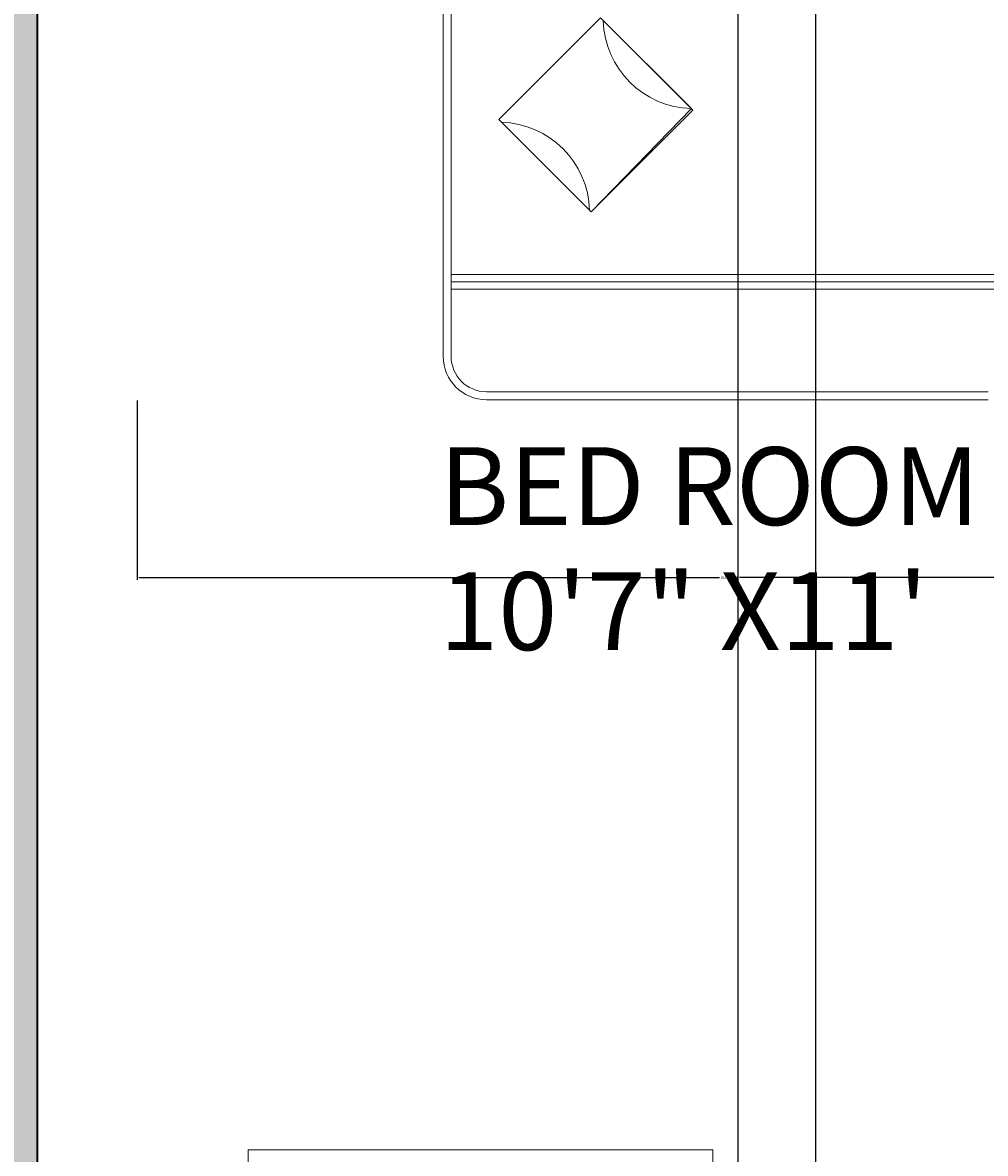
# Model space of a CAD drawing. Units: inches. Extents: x 2070 to 4408, y 1595 to 4269.
# Tile 11 of 20: x 2111 to 2185, y 2150 to 2238. Entities that reach past the tile are written whole.
import ezdxf

# ---------------------------------------------------------------- set-up
doc = ezdxf.new("R2010")
doc.units = ezdxf.units.IN
for name, color, linetype, lineweight in [('A-ANNO-DIMS', 2, 'Continuous', 18), ('A-AREA-IDEN', 7, 'Continuous', 18), ('A-DOOR', 4, 'Continuous', 18), ('A-FURN', 8, 'Continuous', 18), ('A-WALL', 7, 'Continuous', 35)]:
    doc.layers.add(name, color=color, linetype=linetype, lineweight=lineweight)
doc.layers.add('A-WALL-PATT', color=18, linetype='Continuous', lineweight=13, true_color=0x000000)
doc.styles.get("Standard").update_dxf_attribs({"font": 'arial.ttf'})
doc.dimstyles.get("Standard").update_dxf_attribs({"dimtxt": 0.18, "dimasz": 0.18, "dimexe": 0.18, "dimexo": 0.0625, "dimgap": 0.09, "dimtad": 0, "dimtih": 1, "dimtoh": 1, "dimdec": 4, "dimzin": 0, "dimdsep": 46, "dimtxsty": 'Standard', "dimcen": 0.09, "dimadec": 0, "dimazin": 0, "dimtfac": 1, "dimtdec": 4, "dimtofl": 0, "dimtmove": 0, "dimatfit": 3, "dimfxl": 1, "dimtolj": 1, "dimtzin": 0, "dimarcsym": 0})

# ---------------------------------------------------------------- blocks, each defined once
blk = doc.blocks.new('*U3')
for p, q in [((0, 0), (0, 6)), ((40, 0), (40, 6))]:
    blk.add_line(p, q)
blk.add_lwpolyline([(0, 0), (0, -40), (1.75, -40), (1.75, 0)], close=True)
blk.add_arc((0, 0), 40, 270, 0)
blk = doc.blocks.new('A$C18EB7ED0')
for p, q in [((0.7439, 1.8401), (0.7439, 0.1052)), ((0.7632, 1.8401), (0.7632, 0.1052)), ((0.8789, 0.6811), (1.1264, 0.9286)), ((0.8789, 0.6811), (1.1264, 0.9286)), ((1.1264, 0.9286), (1.3473, 0.7077)), ((1.1264, 0.9286), (1.3511, 0.7039)), ((1.3473, 0.7077), (1.1036, 0.4564)), ((1.3511, 0.7039), (1.1036, 0.4564)), ((1.1036, 0.4564), (0.8789, 0.6811)), ((1.1036, 0.4564), (0.8789, 0.6811)), ((0.7632, 0.3045), (2.155, 0.3045)), ((0.7632, 0.2865), (2.155, 0.2865)), ((0.7632, 0.2685), (2.155, 0.2685)), ((0.8491, 0.0193), (2.0691, 0.0193)), ((0.8491, 0), (2.0691, 0))]:
    blk.add_line(p, q)
for centre, radius, start, end in [((1.3534, 0.928), 0.2204, 181.5879, 268.4121), ((0.8795, 0.4541), 0.2204, 1.5879, 88.4121), ((0.8491, 0.1052), 0.1052, 180, 270), ((0.8491, 0.1052), 0.0859, 180, 270)]:
    blk.add_arc(centre, radius, start, end)
blk = doc.blocks.new('*D17')
at = {"layer": 'A-ANNO-DIMS', "color": 0, "lineweight": -2, "transparency": 16777216}
for p, q in [((2119.876, 2208.466), (2119.876, 2194.65)), ((2211.199, 2208.466), (2211.199, 2194.65)), ((2120.056, 2194.83), (2164.767, 2194.83)), ((2211.019, 2194.83), (2166.308, 2194.83))]:
    blk.add_line(p, q, dxfattribs=at)
at = {"layer": 'A-ANNO-DIMS', "color": 0, "transparency": 16777216}
for points in [[(2120.056, 2194.86), (2120.056, 2194.8), (2119.876, 2194.83)], [(2211.019, 2194.86), (2211.019, 2194.8), (2211.199, 2194.83)]]:
    blk.add_solid(points, dxfattribs=at)
at = {"layer": 'Defpoints', "color": 0, "transparency": 16777216}
for p in [(2119.876, 2208.528), (2211.199, 2208.528), (2211.199, 2194.83)]:
    blk.add_point(p, dxfattribs=at)
at = {"layer": 'A-ANNO-DIMS', "color": 0, "transparency": 16777216, "insert": (2165.538, 2194.83), "char_height": 0.18, "attachment_point": 5}
blk.add_mtext('\\A1;BED SET 91', dxfattribs=at)
blk = doc.blocks.new('*D24')
at = {"layer": 'A-ANNO-DIMS', "color": 0, "lineweight": -2, "transparency": 16777216}
for p, q in [((2103.133, 2291.4), (2069.836, 2291.4)), ((2070.016, 2291.22), (2070.016, 1960.081)), ((2070.016, 1628.58), (2070.016, 1959.718)), ((2336.133, 1628.4), (2069.836, 1628.4))]:
    blk.add_line(p, q, dxfattribs=at)
at = {"layer": 'A-ANNO-DIMS', "color": 0, "transparency": 16777216}
for points in [[(2069.986, 2291.22), (2070.046, 2291.22), (2070.016, 2291.4)], [(2069.986, 1628.58), (2070.046, 1628.58), (2070.016, 1628.4)]]:
    blk.add_solid(points, dxfattribs=at)
at = {"layer": 'Defpoints', "color": 0, "transparency": 16777216}
for p in [(2070.016, 2291.4), (2103.196, 2291.4), (2336.196, 1628.4)]:
    blk.add_point(p, dxfattribs=at)
at = {"layer": 'A-ANNO-DIMS', "color": 0, "transparency": 16777216, "insert": (2070.016, 1959.899), "char_height": 0.18, "attachment_point": 5}
blk.add_mtext('\\A1;663', dxfattribs=at)
blk = doc.blocks.new('*D28')
at = {"layer": 'A-ANNO-DIMS', "color": 0, "lineweight": -2, "transparency": 16777216}
for p, q in [((2166.196, 2000.462), (2166.196, 2324.76)), ((2172.196, 2000.462), (2172.196, 2324.76)), ((2166.376, 2324.579), (2169.047, 2324.579)), ((2172.016, 2324.579), (2169.345, 2324.579))]:
    blk.add_line(p, q, dxfattribs=at)
at = {"layer": 'A-ANNO-DIMS', "color": 0, "transparency": 16777216}
for points in [[(2166.376, 2324.61), (2166.376, 2324.55), (2166.196, 2324.579)], [(2172.016, 2324.61), (2172.016, 2324.55), (2172.196, 2324.579)]]:
    blk.add_solid(points, dxfattribs=at)
at = {"layer": 'Defpoints', "color": 0, "transparency": 16777216}
for p in [(2172.196, 2324.579), (2166.196, 2000.399), (2172.196, 2000.399)]:
    blk.add_point(p, dxfattribs=at)
at = {"layer": 'A-ANNO-DIMS', "color": 0, "transparency": 16777216, "insert": (2169.196, 2324.579), "char_height": 0.18, "attachment_point": 5}
blk.add_mtext('\\A1;6', dxfattribs=at)
blk = doc.blocks.new('*D31')
at = {"layer": 'A-ANNO-DIMS', "color": 0, "lineweight": -2, "transparency": 16777216}
for p, q in [((2112.196, 2000.462), (2112.196, 2324.76)), ((2166.196, 2000.462), (2166.196, 2324.76)), ((2112.376, 2324.579), (2138.977, 2324.579)), ((2166.016, 2324.579), (2139.415, 2324.579))]:
    blk.add_line(p, q, dxfattribs=at)
at = {"layer": 'A-ANNO-DIMS', "color": 0, "transparency": 16777216}
for points in [[(2112.376, 2324.61), (2112.376, 2324.55), (2112.196, 2324.579)], [(2166.016, 2324.61), (2166.016, 2324.55), (2166.196, 2324.579)]]:
    blk.add_solid(points, dxfattribs=at)
at = {"layer": 'Defpoints', "color": 0, "transparency": 16777216}
for p in [(2166.196, 2324.579), (2112.196, 2000.399), (2166.196, 2000.399)]:
    blk.add_point(p, dxfattribs=at)
at = {"layer": 'A-ANNO-DIMS', "color": 0, "transparency": 16777216, "insert": (2139.196, 2324.579), "char_height": 0.18, "attachment_point": 5}
blk.add_mtext('\\A1;54', dxfattribs=at)

msp = doc.modelspace()

# ---------------------------------------------------------------- hatches: boundary and pattern name
at = {"layer": 'A-WALL-PATT'}
h = msp.add_hatch(color=256, dxfattribs=at)
h.dxf.hatch_style = 1
h.paths.add_polyline_path([(2346.196, 2218.3995), (2346.196, 2282.3995), (2340.196, 2282.3995), (2340.196, 2212.3995), (2345.5866, 2212.3995), (2346.196, 2212.3995)], flags=0)
h.paths.add_polyline_path([(2245.196, 2282.3995), (2239.196, 2282.3995), (2239.196, 2186.3995), (2244.5866, 2186.3995), (2245.196, 2186.3995)], flags=0)
h.paths.add_polyline_path([(2340.196, 2230.6455), (2245.196, 2230.6455), (2245.196, 2224.6455), (2340.196, 2224.6455)], flags=0)
h.paths.add_polyline_path([(2245.196, 2150.3995), (2239.196, 2150.3995), (2164.4362, 2150.3995), (2164.4362, 2144.3995), (2239.196, 2144.3995), (2239.196, 2086.3995), (2239.196, 2067.2711), (2244.5866, 2067.2711), (2245.196, 2067.2711), (2245.196, 2144.3995)], flags=0)
h.paths.add_polyline_path([(2346.196, 2176.3995), (2340.196, 2176.3995), (2340.196, 2086.3995), (2346.196, 2086.3995), (2346.196, 2125.318)], flags=0)
h.paths.add_polyline_path([(2446.196, 2086.3995), (2346.196, 2086.3995), (2340.196, 2086.3995), (2340.196, 2080.3995), (2446.196, 2080.3995)], flags=0)
h.paths.add_polyline_path([(2455.196, 2291.3995), (2103.196, 2291.3995), (2103.196, 1699.3995), (2336.196, 1699.3995), (2336.196, 1628.3995), (2345.196, 1628.3995), (2446.196, 1628.3995), (2454.8846, 1628.3995), (2454.8846, 1699.3995)])
h.paths.add_polyline_path([(2446.196, 2282.3995), (2446.196, 2218.3995), (2446.196, 2212.3995), (2446.196, 2086.3995), (2446.196, 2080.3995), (2446.196, 1708.3995), (2446.196, 1637.3995), (2345.196, 1637.3995), (2345.196, 1699.3995), (2345.196, 1708.3995), (2336.196, 1708.3995), (2112.196, 1708.3995), (2112.196, 2282.3995), (2239.196, 2282.3995), (2245.196, 2282.3995), (2356.196, 2282.3995)], flags=16)
h.paths.add_polyline_path([(2245.196, 2150.3995), (2245.196, 2144.3995), (2245.196, 2067.2711), (2244.5866, 2067.2711), (2239.196, 2067.2711), (2239.196, 2065.6988), (2203.2929, 2065.6988, 0.4014527), (2239.196, 2031.3337), (2244.5866, 2031.3337), (2245.196, 2031.2711), (2245.196, 1924.1525), (2239.196, 1924.1525), (2239.196, 1922.5803), (2203.2929, 1922.5803, 0.4014527), (2239.196, 1888.2151), (2244.5866, 1888.2151), (2245.196, 1888.1525), (2245.196, 1748.3995), (2339.196, 1748.4621, -0.4014527), (2303.2929, 1782.8272), (2303.2585, 1782.8272), (2303.2585, 1784.3995), (2339.196, 1784.3995), (2339.196, 1877.2067), (2291.196, 1877.2067), (2291.196, 1883.2067), (2291.196, 1946.3995), (2291.196, 1952.3995), (2291.196, 2086.3995), (2297.196, 2086.3995), (2302.196, 2086.3995), (2302.196, 2081.0259), (2303.7633, 2081.0259), (2303.7633, 2080.3995), (2338.0148, 2080.3995, 0.0043713), (2338.0203, 2081.0259), (2338.0203, 2086.3995), (2340.196, 2086.3995), (2340.196, 2176.4621), (2345.5866, 2176.4621, 0.4014527), (2381.4896, 2210.8272), (2345.5866, 2210.8272), (2345.5866, 2212.3995), (2340.196, 2212.3995), (2340.196, 2224.6455), (2245.196, 2224.6455), (2245.196, 2186.3995), (2244.5866, 2186.3995), (2239.196, 2186.3995), (2239.196, 2184.8272), (2203.2929, 2184.8272, 0.4014527), (2239.196, 2150.4621), (2244.5866, 2150.4621)], flags=0)
h.paths.add_polyline_path([(2346.196, 2282.3995), (2346.196, 2218.3995), (2377.1813, 2218.3995), (2377.1813, 2212.3995), (2346.196, 2212.3995), (2345.5866, 2212.3995), (2340.196, 2212.3995), (2340.196, 2224.6455), (2245.196, 2224.6455), (2245.196, 2230.6455), (2245.196, 2282.3995), (2292.696, 2256.5225), (2340.196, 2282.3995)], flags=0)
h.paths.add_polyline_path([(2346.196, 2086.3995), (2340.196, 2086.3995), (2340.196, 2080.3995), (2446.196, 2080.3995), (2431.196, 2016.3995), (2446.196, 1952.3995), (2412.196, 1952.3995), (2412.196, 2080.3995), (2340.196, 2080.3995), (2340.196, 2086.3995), (2340.196, 2176.3995), (2346.196, 2176.3995), (2346.196, 2125.318)], flags=0)
h.paths.add_polyline_path([(2186.508, 2270.0471, -0.0375529), (2186.9712, 2269.8581), (2186.9164, 2270.112, -0.0275912)], flags=0)
h.paths.add_polyline_path([(2183.955, 2273.7766, 1), (2188.2945, 2273.7766, 1)], flags=0)
h.paths.add_polyline_path([(2142.5261, 2274.6158, -0.0370754), (2142.5672, 2275.1696), (2142.5672, 2276.826), (2119.8759, 2276.826), (2119.8759, 2263.0962), (2140.4332, 2263.0962), (2142.5672, 2263.0962), (2142.5672, 2274.0621, -0.0370754)], flags=0)
h.paths.add_polyline_path([(2209.8974, 2263.0962), (2209.8974, 2262.2079), (2190.8042, 2262.2079), (2190.8042, 2263.0962)], flags=0)
h.paths.add_polyline_path([(2210.6382, 2276.1833), (2210.6382, 2263.9844), (2190.2185, 2263.9844), (2190.2185, 2276.1833)], flags=0)
h.paths.add_polyline_path([(2188.4362, 2273.7766, -1), (2183.8133, 2273.7766, -1)], flags=0)
h.paths.add_polyline_path([(2245.196, 2150.3995), (2245.196, 2144.3995), (2245.196, 2067.2711), (2239.196, 2067.2711), (2239.196, 2080.3995), (2172.196, 2080.3995), (2172.196, 2000.3995), (2239.196, 2000.3995), (2239.196, 1940.3995), (2159.0187, 1940.3995), (2123.0187, 1940.3995), (2112.196, 1940.3995), (2112.196, 1946.3995), (2123.0187, 1946.3995), (2123.0187, 1982.2238), (2124.586, 1982.2238), (2124.586, 1982.1895, -0.4014527), (2158.8429, 1946.3995), (2159.0187, 1946.3995), (2239.196, 1946.3995), (2239.196, 1994.3995), (2112.196, 1994.3995), (2112.196, 2000.3995), (2139.196, 2040.3995), (2112.196, 2080.3995), (2112.196, 2086.3995), (2239.196, 2086.3995), (2239.196, 2144.3995), (2209.5809, 2144.3995), (2209.5809, 2136.3995), (2203.0809, 2136.3995), (2205.0809, 2130.3996, -0.7025712), (2199.081, 2116.3995, -0.7025621), (2193.0809, 2130.3994), (2195.0809, 2136.3995), (2192.0809, 2136.3995), (2192.0809, 2134.8995), (2189.0809, 2134.8995), (2189.0809, 2135.8995), (2191.0809, 2135.8995), (2191.0809, 2136.3995), (2188.5809, 2136.3995), (2188.5809, 2144.3995), (2164.2481, 2144.3995, -0.3938585), (2130.0035, 2109.5491), (2130.0035, 2109.5147), (2128.4362, 2109.5147), (2128.4362, 2144.3995), (2112.196, 2144.3995), (2112.196, 2150.3995), (2128.4362, 2150.3995), (2128.4362, 2150.7127), (2164.4362, 2150.7127), (2164.4362, 2150.3995), (2239.196, 2150.3995)], flags=0)
h.paths.add_polyline_path([(2188.2075, 2266.8735), (2188.2075, 2211.8632, -0.4142136), (2185.4833, 2209.1391), (2146.7995, 2209.1391, -0.4142136), (2144.0754, 2211.8632), (2144.0754, 2266.8735, -0.4142136), (2146.7995, 2269.5976), (2185.4833, 2269.5976, -0.4142136)], flags=0)
h.paths.add_polyline_path([(2185.0844, 2273.7766, -1), (2187.1651, 2273.7766, -1)], flags=0)
h.paths.add_polyline_path([(2182.0486, 2259.2932), (2168.0953, 2259.2932), (2168.0953, 2260.8424), (2163.7261, 2260.8424), (2163.7261, 2259.2932), (2149.7727, 2259.2932), (2149.7727, 2266.3352), (2163.7261, 2266.3352), (2163.7261, 2261.9839), (2168.0953, 2261.9839), (2168.0953, 2266.3352), (2182.0486, 2266.3352)], flags=0)
h.paths.add_polyline_path([(2148.2585, 2250.2051), (2153.0615, 2241.8861, 0.3980705)], flags=0)
h.paths.add_polyline_path([(2162.7572, 2247.2885), (2153.1461, 2241.7396), (2148.1083, 2250.4653), (2157.7194, 2256.0142)], flags=0)
h.paths.add_polyline_path([(2162.6726, 2247.4351, -0.392862), (2157.8415, 2255.6313), (2157.6431, 2255.6313), (2157.8696, 2255.7541)], flags=0)
h.paths.add_polyline_path([(2164.2604, 2145.339), (2164.4362, 2144.3995), (2164.4362, 2150.3995), (2164.2604, 2150.7127)], flags=0)
h.paths.add_polyline_path([(2208.5809, 2142.6495), (2208.5809, 2138.3995, -0.4142136), (2207.8309, 2137.3995), (2190.5809, 2137.3995, -0.4142136), (2189.5809, 2138.1495), (2189.5809, 2142.3995, -0.4142136), (2190.3309, 2143.3995), (2207.5809, 2143.3995, -0.4142136)], flags=0)
h.paths.add_polyline_path([(2147.957, 2229.9119), (2154.7494, 2223.1195, 0.3980705)], flags=0)
h.paths.add_polyline_path([(2162.7165, 2230.8473), (2154.8691, 2222.9998), (2147.7446, 2230.1244), (2155.592, 2237.9718)], flags=0)
h.paths.add_polyline_path([(2162.5969, 2230.9669, -0.3980705), (2155.8044, 2237.7594)], flags=0)
h.paths.add_polyline_path([(2391.8776, 2049.9192), (2408.5766, 2049.9192), (2408.5766, 2033.2202), (2408.5766, 1983.123), (2408.5766, 1966.4239), (2391.8776, 1966.4239), (2391.8776, 1983.123), (2341.7804, 1983.123), (2341.7804, 2033.2202), (2391.8776, 2033.2202)], flags=0)
h.paths.add_polyline_path([(2144.1055, 2274.6158, 1), (2148.445, 2274.6158, 1)], flags=0)
h.paths.add_polyline_path([(2148.5867, 2274.6158, -1), (2143.9638, 2274.6158, -1)], flags=0)
h.paths.add_polyline_path([(2145.2349, 2274.6158, -1), (2147.3156, 2274.6158, -1)], flags=0)
edge = h.paths.add_edge_path(flags=0)
edge.add_ellipse((2400.5951, 2040.9436), major_axis=(-4.5109, 0), ratio=0.9754478, start_angle=180, end_angle=270, ccw=False)
edge.add_ellipse((2400.5951, 2040.9436), major_axis=(-4.5109, 0), ratio=0.9754478, start_angle=90, end_angle=180, ccw=False)
edge.add_ellipse((2400.5951, 2040.9436), major_axis=(-4.5109, 0), ratio=0.9754478, start_angle=0, end_angle=90, ccw=False)
edge.add_ellipse((2400.5951, 2040.9436), major_axis=(-4.5109, 0), ratio=0.9754478, start_angle=270, end_angle=360, ccw=False)
h.paths.add_polyline_path([(2199.0809, 2117.3995, -0.7345297), (2195.0809, 2130.3995), (2203.081, 2130.3995, -0.7345333)], flags=0)
h.paths.add_polyline_path([(2141.9147, 2276.0353), (2141.9147, 2263.9844), (2120.4685, 2263.9844), (2120.4685, 2276.0353)], flags=0)
h.paths.add_polyline_path([(2138.4481, 2273.4072), (2138.4481, 2266.7226), (2133.2801, 2266.7226), (2133.2801, 2273.4072)], flags=0)
h.paths.add_polyline_path([(2137.9691, 2272.9175), (2137.9691, 2272.204), (2135.4229, 2272.204), (2135.4229, 2271.6329), (2135.3221, 2270.1051), (2135.3221, 2269.0265), (2135.4229, 2268.6811), (2135.4229, 2267.2011), (2133.7212, 2267.2011), (2133.7212, 2268.6811), (2133.7983, 2269.9587), (2133.7983, 2271.2758), (2133.7212, 2271.6329), (2133.7212, 2273.0065), (2135.717, 2273.0065), (2135.717, 2272.9175)], flags=0)
h.paths.add_polyline_path([(2137.9215, 2271.8264), (2137.9215, 2271.3786), (2137.5182, 2271.3786), (2136.9355, 2271.3786), (2136.3529, 2271.3786), (2135.7703, 2271.3786), (2135.7703, 2271.8264), (2136.1736, 2271.8264), (2136.7562, 2271.8264), (2137.3389, 2271.8264)], flags=0)
h.paths.add_polyline_path([(2137.9215, 2271.692), (2137.5182, 2271.692), (2136.9355, 2271.513), (2137.3389, 2271.513)], flags=0)
h.paths.add_polyline_path([(2136.3529, 2271.692), (2135.7703, 2271.513), (2136.1736, 2271.513), (2136.7562, 2271.692)], flags=0)
h.paths.add_polyline_path([(2137.9215, 2271.513), (2137.5182, 2271.513), (2136.7562, 2271.747), (2136.7562, 2271.692), (2137.3389, 2271.692)], flags=0)
h.paths.add_polyline_path([(2137.8207, 2270.4664), (2137.8207, 2270.0971), (2137.8207, 2269.627), (2137.8207, 2269.1569), (2137.8207, 2268.6868), (2137.3837, 2268.6868), (2136.6442, 2268.6868), (2135.9271, 2268.6868), (2135.9271, 2269.0562), (2135.9271, 2269.5263), (2135.9271, 2269.9963), (2135.9271, 2270.4664), (2136.3641, 2270.4664), (2137.0812, 2270.4664)], flags=0)
h.paths.add_polyline_path([(2137.3837, 2269.627), (2137.8207, 2269.627), (2137.8207, 2269.5263), (2137.3837, 2269.5263), (2137.3837, 2269.1569), (2137.8207, 2269.1569), (2137.3837, 2269.0562), (2137.3837, 2268.6868), (2137.0812, 2268.6868), (2137.0812, 2269.0562), (2136.6442, 2269.0562), (2136.6442, 2268.6868), (2136.3641, 2268.6868), (2136.3641, 2269.0562), (2135.9271, 2269.0562), (2135.9271, 2269.1569), (2136.3641, 2269.1569), (2136.3641, 2269.5263), (2135.9271, 2269.5263), (2135.9271, 2269.627), (2136.3641, 2269.627), (2136.3641, 2269.9963), (2135.9271, 2269.9963), (2136.3641, 2270.0971), (2136.3641, 2270.4664), (2136.6442, 2270.4664), (2136.6442, 2270.0971), (2137.0812, 2270.0971), (2137.0812, 2270.4664), (2137.3837, 2270.4664), (2137.3837, 2270.0971), (2137.8207, 2270.0971), (2137.3837, 2269.9963)], flags=0)
h.paths.add_polyline_path([(2137.5182, 2271.8264), (2137.5182, 2271.692), (2137.3389, 2271.3786), (2137.3389, 2271.513)], flags=0)
h.paths.add_polyline_path([(2137.8179, 2267.8138), (2137.8179, 2267.6879), (2137.1876, 2267.6879), (2136.4733, 2267.6879), (2135.759, 2267.6879), (2135.759, 2267.8138), (2136.3893, 2267.8138), (2137.1036, 2267.8138)], flags=0)
h.paths.add_polyline_path([(2137.0812, 2269.9963), (2137.0812, 2269.627), (2137.0812, 2269.1569), (2136.6442, 2269.1569), (2136.6442, 2269.5263), (2136.6442, 2269.9963)], flags=0)
h.paths.add_polyline_path([(2136.3529, 2271.8264), (2136.3529, 2271.692), (2136.1736, 2271.3786), (2136.1736, 2271.513)], flags=0)
h.paths.add_polyline_path([(2136.4733, 2267.8138), (2136.4733, 2267.6879), (2136.3893, 2267.6879), (2136.3893, 2267.8138)], flags=0)
h.paths.add_polyline_path([(2407.9087, 2032.5522), (2407.9087, 1983.7909), (2359.81, 1983.7909, -0.0091279), (2359.0575, 1983.7909), (2342.4483, 1983.7909), (2342.4483, 2032.5522)], flags=0)
h.paths.add_polyline_path([(2389.1838, 2023.1358), (2353.7856, 2023.1358), (2353.7856, 1985.4867, -0.0921038), (2350.2788, 1988.655), (2350.2788, 2026.6426), (2389.1838, 2026.6426)], flags=0)
h.paths.add_polyline_path([(2352.6166, 2024.3048), (2351.4477, 2024.3048), (2351.4477, 2025.4737), (2352.6166, 2025.4737)], flags=0)
h.paths.add_polyline_path([(2399.6319, 2026.7589), (2404.3661, 2026.7589, -0.4142136), (2407.0379, 2024.087), (2407.0379, 2013.4908, -0.4142136), (2404.3661, 2010.819), (2399.6319, 2010.819, -0.4142136), (2396.96, 2013.4908), (2396.96, 2024.087, -0.4142136)], flags=0)
h.paths.add_polyline_path([(2399.6319, 2026.0909), (2404.3661, 2026.0909, -0.4142136), (2406.37, 2024.087), (2406.37, 2013.4908, -0.4142136), (2404.3661, 2011.487), (2399.6319, 2011.487, -0.4142136), (2397.628, 2013.4908), (2397.628, 2024.087, -0.4142136)], flags=0)
h.paths.add_polyline_path([(2399.6319, 2002.3217), (2404.3661, 2002.3217, -0.4142136), (2407.0379, 1999.6498), (2407.0379, 1989.0536, -0.4142136), (2404.3661, 1986.3818), (2399.6319, 1986.3818, -0.4142136), (2396.96, 1989.0536), (2396.96, 1999.6498, -0.4142136)], flags=0)
h.paths.add_polyline_path([(2399.6319, 2001.6537), (2404.3661, 2001.6537, -0.4142136), (2406.37, 1999.6498), (2406.37, 1989.0536, -0.4142136), (2404.3661, 1987.0497), (2399.6319, 1987.0497, -0.4142136), (2397.628, 1989.0536), (2397.628, 1999.6498, -0.4142136)], flags=0)
edge = h.paths.add_edge_path(flags=0)
edge.add_ellipse((2400.5951, 1975.3996), major_axis=(-4.5109, 0), ratio=0.9754478, start_angle=-180, end_angle=-90, ccw=False)
edge.add_ellipse((2400.5951, 1975.3996), major_axis=(-4.5109, 0), ratio=0.9754478, start_angle=90, end_angle=180, ccw=False)
edge.add_ellipse((2400.5951, 1975.3996), major_axis=(-4.5109, 0), ratio=0.9754478, start_angle=0, end_angle=90, ccw=False)
edge.add_ellipse((2400.5951, 1975.3996), major_axis=(-4.5109, 0), ratio=0.9754478, start_angle=-90, end_angle=0, ccw=False)
h.paths.add_polyline_path([(2345.196, 1910.3995), (2366.4386, 1910.3995), (2366.4386, 1925.4555), (2392.3856, 1925.4555), (2392.3856, 1933.5025), (2400.1399, 1925.4555), (2392.3856, 1919.8795), (2392.3856, 1925.4555), (2366.4386, 1925.4555), (2366.4386, 1910.3995), (2381.196, 1910.3995), (2405.196, 1910.3995), (2405.196, 1898.3995), (2446.196, 1898.3995), (2446.196, 1886.3995), (2405.196, 1886.3995), (2405.196, 1874.3995), (2446.196, 1874.3995), (2446.196, 1862.3995), (2405.196, 1862.3995), (2405.196, 1850.3995), (2446.196, 1850.3995), (2446.196, 1838.3995), (2405.196, 1838.3995), (2405.196, 1826.3995), (2446.196, 1826.3995), (2446.196, 1814.3995), (2405.196, 1814.3995), (2405.196, 1802.3995), (2446.196, 1802.3995), (2446.196, 1798.3995), (2446.196, 1792.3995), (2405.196, 1792.3995), (2405.196, 1910.3995), (2381.196, 1910.3995), (2381.196, 1792.3995), (2345.196, 1792.3995)], flags=0)
h.paths.add_polyline_path([(2333.0944, 1863.3993, -0.4142136), (2334.7225, 1861.7712), (2334.7225, 1859.329), (2335.2653, 1859.329, -0.4142136), (2337.4361, 1857.1582), (2337.4361, 1843.862, -0.4142136), (2335.2653, 1841.6911, -0.4142136), (2337.4361, 1839.5203), (2337.4361, 1827.5808, -0.4142136), (2335.2653, 1825.41, -0.4142136), (2337.4361, 1823.2392), (2337.4361, 1808.5862, -0.4142136), (2335.2653, 1806.4153), (2334.7225, 1806.4153), (2334.7225, 1803.9732, -0.4142136), (2333.0944, 1802.3451), (2317.356, 1802.3451), (2317.0846, 1802.3451, -0.4142136), (2315.7279, 1803.7018), (2315.7279, 1803.8646), (2313.8284, 1803.8646, -0.4142136), (2311.6576, 1806.0354), (2311.6576, 1823.2015, -0.395976), (2313.6834, 1825.3765, -0.433848), (2311.6576, 1827.2718), (2311.6576, 1839.761, -0.4142136), (2313.5571, 1841.6604), (2313.8284, 1841.6604), (2333.8159, 1841.6604, -0.0421362), (2334.1798, 1841.6911, -0.4142136), (2332.009, 1843.862), (2332.009, 1857.1582, -0.4142136), (2334.1798, 1859.329), (2317.356, 1859.329), (2317.0846, 1859.329, -0.4142136), (2315.7279, 1860.6858), (2315.7279, 1862.0426, -0.4142136), (2317.0846, 1863.3993), (2317.356, 1863.3993)], flags=0)
h.paths.add_polyline_path([(2208.8475, 1848.9818), (2208.8475, 1840.9741, -0.4142136), (2207.0458, 1839.1724), (2206.5453, 1839.1721), (2206.5453, 1838.7218, -0.4098586), (2204.7704, 1836.9203), (2183.7501, 1836.9203, -0.418582), (2181.9216, 1838.7218), (2181.9216, 1839.1721), (2181.421, 1839.1724, -0.4142136), (2179.6193, 1840.9741), (2179.6193, 1848.6817, -0.4406442), (2185.1126, 1854.9874), (2203.3852, 1854.9874, -0.4570796)], flags=0)
h.paths.add_polyline_path([(2204.243, 1848.4815), (2204.243, 1848.4815, 0.4172533), (2202.2204, 1850.4833), (2186.2049, 1850.4833, 0.4111805), (2184.2237, 1848.4815), (2184.2237, 1848.4815, -0.4111807), (2186.2049, 1850.4833), (2202.2204, 1850.4833, -0.4172531)], flags=0)
h.paths.add_polyline_path([(2234.7177, 1830.228), (2234.7176, 1781.6047, -0.4142136), (2233.4381, 1780.3252), (2218.6064, 1780.3252, -0.4142136), (2217.8387, 1781.0929), (2217.8387, 1783.3961, -0.4142136), (2218.6064, 1784.1639), (2218.6065, 1796.9595, -0.4142136), (2219.886, 1798.239, -0.4142136), (2218.6065, 1799.5186), (2218.6065, 1812.3142, -0.4142136), (2219.8861, 1813.5938, -0.4142136), (2218.6065, 1814.8733), (2218.6065, 1827.6689, -0.4142136), (2217.8388, 1828.4367), (2217.8388, 1830.7399, -0.4142136), (2218.6065, 1831.5076), (2233.4382, 1831.5076, -0.4142136)], flags=0)
h.paths.add_polyline_path([(2230.6344, 1827.6689, -0.4142136), (2231.4021, 1826.9012), (2231.4021, 1784.9316, -0.4142136), (2230.6343, 1784.1639), (2221.1853, 1784.1639), (2221.1853, 1827.6689)], flags=0)
h.paths.add_polyline_path([(2222.7208, 1798.239), (2221.6971, 1798.239), (2221.6971, 1813.5938), (2222.7208, 1813.5938)], flags=0)
h.paths.add_polyline_path([(2206.5453, 1773.935), (2206.5453, 1773.4848), (2206.9457, 1773.4848), (2207.0458, 1773.4845, -0.4142136), (2208.8475, 1771.6827), (2208.8475, 1763.675, -0.4422243), (2203.6505, 1757.6695), (2185.3851, 1757.6695, -0.455084), (2179.6193, 1763.9752), (2179.6193, 1771.6827, -0.4142136), (2181.421, 1773.4845), (2181.421, 1773.4848), (2181.9216, 1773.4848), (2181.9216, 1773.935, -0.4098586), (2183.6965, 1775.7366), (2204.7167, 1775.7366, -0.418582)], flags=0)
h.paths.add_polyline_path([(2202.2619, 1762.1736), (2186.2464, 1762.1736, -0.4172531), (2184.2237, 1764.1754), (2184.2237, 1764.1754, 0.4172533), (2186.2464, 1762.1736), (2202.2619, 1762.1736, 0.4111805), (2204.243, 1764.1754), (2204.243, 1764.1754, -0.4111807)], flags=0)
h.paths.add_polyline_path([(2313.0034, 1713.1906), (2312.997, 1713.1697), (2313.0123, 1713.1612)], flags=0)
h.paths.add_polyline_path([(2305.7314, 1721.0488), (2305.6257, 1721.1994), (2305.4853, 1721.084)], flags=0)
h.paths.add_polyline_path([(2307.5562, 1726.1427), (2307.6186, 1726.1026), (2307.5737, 1726.0477), (2308.5692, 1720.6434), (2310.5345, 1721.2985), (2310.5721, 1721.411), (2310.6958, 1721.3523), (2313.8453, 1722.4021), (2314.9351, 1723.8033), (2314.9294, 1723.9165), (2315.0028, 1723.8903), (2313.874, 1722.4389), (2313.8697, 1722.4102), (2308.5692, 1720.6434), (2308.9864, 1720.122), (2309.0665, 1720.0971), (2309.053, 1720.0387), (2310.9235, 1717.7005), (2311.4182, 1717.6259), (2311.2918, 1717.2402), (2312.0655, 1716.2731), (2312.1081, 1716.2606), (2312.0969, 1716.2339), (2308.5692, 1720.6434), (2305.2249, 1717.745), (2305.232, 1717.704), (2305.1665, 1717.6944), (2308.5692, 1720.6434)], flags=0)
h.paths.add_polyline_path([(2288.2072, 1714.3431), (2288.2008, 1714.3222), (2288.216, 1714.3137)], flags=0)
h.paths.add_polyline_path([(2280.9352, 1722.2013), (2280.8295, 1722.3519), (2280.689, 1722.2365)], flags=0)
h.paths.add_polyline_path([(2282.76, 1727.2952), (2282.8224, 1727.2551), (2282.7775, 1727.2002), (2283.773, 1721.7959), (2285.7383, 1722.451), (2285.7759, 1722.5635), (2285.8995, 1722.5048), (2289.0491, 1723.5546), (2290.1389, 1724.9558), (2290.1332, 1725.069), (2290.2065, 1725.0428), (2289.0777, 1723.5915), (2289.0735, 1723.5628), (2283.773, 1721.7959), (2284.1901, 1721.2745), (2284.2703, 1721.2496), (2284.2567, 1721.1913), (2286.1273, 1718.8531), (2286.622, 1718.7785), (2286.4956, 1718.3927), (2287.2692, 1717.4256), (2287.3119, 1717.4131), (2287.3006, 1717.3864), (2283.773, 1721.7959), (2280.4286, 1718.8975), (2280.4357, 1718.8565), (2280.3703, 1718.8469), (2283.773, 1721.7959)], flags=0)
h.paths.add_polyline_path([(2302.0672, 1721.8694), (2301.8205, 1721.8572), (2301.7578, 1722.1787), (2299.415, 1724.5215), (2299.103, 1724.4694), (2299.0662, 1724.8703)], flags=0)
h.paths.add_polyline_path([(2264.5643, 1715.4956), (2264.5579, 1715.4747), (2264.5731, 1715.4662)], flags=0)
h.paths.add_polyline_path([(2257.2923, 1723.3538), (2257.1865, 1723.5044), (2257.0461, 1723.389)], flags=0)
h.paths.add_polyline_path([(2259.117, 1728.4477), (2259.1795, 1728.4077), (2259.1345, 1728.3527), (2260.13, 1722.9484), (2262.0954, 1723.6036), (2262.133, 1723.716), (2262.2566, 1723.6573), (2265.4061, 1724.7071), (2266.4959, 1726.1083), (2266.4902, 1726.2215), (2266.5636, 1726.1953), (2265.4348, 1724.744), (2265.4305, 1724.7153), (2260.13, 1722.9484), (2260.5472, 1722.427), (2260.6273, 1722.4022), (2260.6138, 1722.3438), (2262.4843, 1720.0056), (2262.979, 1719.931), (2262.8526, 1719.5452), (2263.6263, 1718.5781), (2263.6689, 1718.5656), (2263.6577, 1718.5389), (2260.13, 1722.9484), (2256.7857, 1720.05), (2256.7928, 1720.009), (2256.7273, 1719.9994), (2260.13, 1722.9484)], flags=0)
h.paths.add_polyline_path([(2277.2709, 1723.0219), (2277.0243, 1723.0097), (2276.9616, 1723.3312), (2274.6187, 1725.6741), (2274.3067, 1725.6219), (2274.27, 1726.0228)], flags=0)
h.paths.add_polyline_path([(2253.628, 1724.1744), (2253.3814, 1724.1622), (2253.3186, 1724.4838), (2250.9758, 1726.8266), (2250.6638, 1726.7744), (2250.627, 1727.1753)], flags=0)
h.paths.add_polyline_path([(2161.9194, 1715.4956), (2161.913, 1715.4747), (2161.9282, 1715.4662)], flags=0)
h.paths.add_polyline_path([(2154.6474, 1723.3538), (2154.5416, 1723.5044), (2154.4012, 1723.389)], flags=0)
h.paths.add_polyline_path([(2162.7899, 1724.744), (2162.7856, 1724.7153), (2157.4851, 1722.9484), (2157.9023, 1722.427), (2157.9824, 1722.4022), (2157.9689, 1722.3438), (2159.8394, 1720.0056), (2160.3341, 1719.931), (2160.2078, 1719.5452), (2160.9814, 1718.5781), (2161.024, 1718.5656), (2161.0128, 1718.5389), (2157.4851, 1722.9484), (2154.1408, 1720.05), (2154.1479, 1720.009), (2154.0824, 1719.9994), (2157.4851, 1722.9484), (2156.4721, 1728.4477), (2156.5346, 1728.4077), (2156.4896, 1728.3527), (2157.4851, 1722.9484), (2159.4505, 1723.6036), (2159.4881, 1723.716), (2159.6117, 1723.6573), (2162.7612, 1724.7071), (2163.851, 1726.1083), (2163.8453, 1726.2215), (2163.9187, 1726.1953)], flags=0)
h.paths.add_polyline_path([(2150.9831, 1724.1744), (2150.7365, 1724.1622), (2150.6738, 1724.4838), (2148.3309, 1726.8266), (2148.0189, 1726.7744), (2147.9822, 1727.1753)], flags=0)
h.paths.add_polyline_path([(2132.5099, 1716.6482), (2132.5035, 1716.6272), (2132.5187, 1716.6187)], flags=0)
h.paths.add_polyline_path([(2125.2379, 1724.5064), (2125.1322, 1724.6569), (2124.9917, 1724.5415)], flags=0)
h.paths.add_polyline_path([(2133.3804, 1725.8965), (2133.3762, 1725.8678), (2128.0757, 1724.101), (2128.4928, 1723.5795), (2128.5729, 1723.5547), (2128.5594, 1723.4963), (2130.43, 1721.1581), (2130.9246, 1721.0835), (2130.7983, 1720.6977), (2131.5719, 1719.7306), (2131.6146, 1719.7181), (2131.6033, 1719.6914), (2128.0757, 1724.101), (2124.7313, 1721.2025), (2124.7384, 1721.1615), (2124.6729, 1721.1519), (2128.0757, 1724.101), (2127.0626, 1729.6002), (2127.1251, 1729.5602), (2127.0801, 1729.5052), (2128.0757, 1724.101), (2130.041, 1724.7561), (2130.0786, 1724.8685), (2130.2022, 1724.8098), (2133.3517, 1725.8597), (2134.4415, 1727.2608), (2134.4358, 1727.3741), (2134.5092, 1727.3478)], flags=0)
h.paths.add_polyline_path([(2121.5736, 1725.3269), (2121.327, 1725.3148), (2121.2643, 1725.6363), (2118.9214, 1727.9791), (2118.6094, 1727.9269), (2118.5727, 1728.3279)], flags=0)
h.paths.add_polyline_path([(2433.3904, 1646.406), (2433.384, 1646.3851), (2433.3992, 1646.3766)], flags=0)
h.paths.add_polyline_path([(2426.1184, 1654.2642), (2426.0127, 1654.4148), (2425.8722, 1654.2994)], flags=0)
h.paths.add_polyline_path([(2427.9432, 1659.3581), (2428.0056, 1659.318), (2427.9606, 1659.2631), (2428.9562, 1653.8588), (2430.9215, 1654.514), (2430.9591, 1654.6264), (2431.0827, 1654.5677), (2434.2323, 1655.6175), (2435.322, 1657.0187), (2435.3163, 1657.1319), (2435.3897, 1657.1057), (2434.2609, 1655.6544), (2434.2567, 1655.6257), (2428.9562, 1653.8588), (2429.3733, 1653.3374), (2429.4534, 1653.3126), (2429.4399, 1653.2542), (2431.3105, 1650.916), (2431.8051, 1650.8414), (2431.6788, 1650.4556), (2432.4524, 1649.4885), (2432.4951, 1649.476), (2432.4838, 1649.4493), (2428.9562, 1653.8588), (2425.6118, 1650.9604), (2425.6189, 1650.9194), (2425.5535, 1650.9098), (2428.9562, 1653.8588)], flags=0)
h.paths.add_polyline_path([(2376.63, 1645.4912), (2376.6236, 1645.4703), (2376.6388, 1645.4617)], flags=0)
h.paths.add_polyline_path([(2369.358, 1653.3494), (2369.2523, 1653.5), (2369.1118, 1653.3845)], flags=0)
h.paths.add_polyline_path([(2371.1828, 1658.4432), (2371.2452, 1658.4032), (2371.2003, 1658.3482), (2372.1958, 1652.944), (2374.1611, 1653.5991), (2374.1987, 1653.7116), (2374.3224, 1653.6528), (2377.4719, 1654.7027), (2378.5617, 1656.1038), (2378.556, 1656.2171), (2378.6293, 1656.1908), (2377.5005, 1654.7395), (2377.4963, 1654.7108), (2372.1958, 1652.944), (2372.6129, 1652.4225), (2372.6931, 1652.3977), (2372.6795, 1652.3393), (2374.5501, 1650.0011), (2375.0448, 1649.9265), (2374.9184, 1649.5407), (2375.692, 1648.5737), (2375.7347, 1648.5611), (2375.7234, 1648.5344), (2372.1958, 1652.944), (2368.8514, 1650.0456), (2368.8586, 1650.0046), (2368.7931, 1649.995), (2372.1958, 1652.944)], flags=0)
h.paths.add_polyline_path([(2404.0947, 1645.0338), (2404.0883, 1645.0128), (2404.1035, 1645.0043)], flags=0)
h.paths.add_polyline_path([(2396.8227, 1652.892), (2396.717, 1653.0425), (2396.5765, 1652.9271)], flags=0)
h.paths.add_polyline_path([(2398.6475, 1657.9858), (2398.7099, 1657.9458), (2398.665, 1657.8908), (2399.6605, 1652.4866), (2401.6258, 1653.1417), (2401.6634, 1653.2541), (2401.7871, 1653.1954), (2404.9366, 1654.2453), (2406.0264, 1655.6464), (2406.0207, 1655.7596), (2406.094, 1655.7334), (2404.9652, 1654.2821), (2404.961, 1654.2534), (2399.6605, 1652.4866), (2400.0776, 1651.9651), (2400.1578, 1651.9403), (2400.1442, 1651.8819), (2402.0148, 1649.5437), (2402.5095, 1649.4691), (2402.3831, 1649.0833), (2403.1567, 1648.1162), (2403.1994, 1648.1037), (2403.1881, 1648.077), (2399.6605, 1652.4866), (2396.3162, 1649.5881), (2396.3233, 1649.5471), (2396.2578, 1649.5375), (2399.6605, 1652.4866)], flags=0)
h.paths.add_polyline_path([(2419.4532, 1658.0857), (2422.4541, 1655.0848), (2422.2075, 1655.0726), (2422.1448, 1655.3941), (2419.8019, 1657.737), (2419.4899, 1657.6848)], flags=0)
h.paths.add_polyline_path([(2390.1575, 1656.7135), (2393.1584, 1653.7125), (2392.9118, 1653.7004), (2392.8491, 1654.0219), (2390.5063, 1656.3647), (2390.1943, 1656.3125)], flags=0)
h.paths.add_polyline_path([(2362.6928, 1657.1709), (2365.6937, 1654.1699), (2365.4471, 1654.1578), (2365.3844, 1654.4793), (2363.0416, 1656.8221), (2362.7295, 1656.77)], flags=0)
h.paths.add_polyline_path([(2419.9523, 2037.8601), (2440.2872, 2037.8601), (2440.2872, 2047.1732), (2419.9523, 2047.1732)], flags=8)
h.paths.add_polyline_path([(2370.186, 1698.9005), (2413.6287, 1698.9005), (2413.6287, 1708.0908), (2370.186, 1708.0908)], flags=8)
h.paths.add_polyline_path([(2370.1656, 1708.5185), (2430.0857, 1708.5185), (2430.0857, 1717.8316), (2370.1656, 1717.8316)], flags=8)
h.paths.add_polyline_path([(2254.1469, 1788.1883), (2302.2471, 1788.1883), (2302.2471, 1797.3786), (2254.1469, 1797.3786)], flags=8)
h.paths.add_polyline_path([(2254.1264, 1797.8063), (2326.1448, 1797.8063), (2326.1448, 1807.1194), (2254.1264, 1807.1194)], flags=8)
h.paths.add_polyline_path([(2300.08, 1914.5069), (2338.861, 1914.5069), (2338.861, 1923.6972), (2300.08, 1923.6972)], flags=8)
h.paths.add_polyline_path([(2300.0595, 1924.1249), (2331.5882, 1924.1249), (2331.5882, 1933.438), (2300.0595, 1933.438)], flags=8)
h.paths.add_polyline_path([(2176.6905, 1716.4567), (2224.1441, 1716.4567), (2224.1441, 1725.647), (2176.6905, 1725.647)], flags=8)
h.paths.add_polyline_path([(2176.67, 1726.0747), (2245.9176, 1726.0747), (2245.9176, 1735.3878), (2176.67, 1735.3878)], flags=8)
h.paths.add_polyline_path([(2339.997, 2039.7696), (2388.1034, 2039.7696), (2388.1034, 2048.9661), (2339.997, 2048.9661)], flags=8)
h.paths.add_polyline_path([(2339.9776, 2049.3928), (2388.7204, 2049.3928), (2388.7204, 2058.7059), (2339.9776, 2058.7059)], flags=8)
h.paths.add_polyline_path([(2366.0063, 2161.3825), (2409.449, 2161.3825), (2409.449, 2170.5728), (2366.0063, 2170.5728)], flags=8)
h.paths.add_polyline_path([(2365.9868, 2171.0016), (2405.879, 2171.0016), (2405.879, 2180.3085), (2365.9868, 2180.3085)], flags=8)
h.paths.add_polyline_path([(2366.0102, 2247.0726), (2407.12, 2247.0726), (2407.12, 2256.263), (2366.0102, 2256.263)], flags=8)
h.paths.add_polyline_path([(2365.9897, 2256.6906), (2397.9686, 2256.6906), (2397.9686, 2266.0037), (2365.9897, 2266.0037)], flags=8)
h.paths.add_polyline_path([(2271.8465, 2102.7885), (2307.6541, 2102.7885), (2307.6541, 2111.9849), (2271.8465, 2111.9849)], flags=8)
h.paths.add_polyline_path([(2271.8281, 2112.4126), (2304.2673, 2112.4126), (2304.2673, 2121.7196), (2271.8281, 2121.7196)], flags=8)
h.paths.add_polyline_path([(2141.6408, 2187.5934), (2182.108, 2187.5934), (2182.108, 2196.7837), (2141.6408, 2196.7837)], flags=8)
h.paths.add_polyline_path([(2141.6203, 2197.2114), (2190.3631, 2197.2114), (2190.3631, 2206.5245), (2141.6203, 2206.5245)], flags=8)
h.paths.add_polyline_path([(2165.7271, 2103.039), (2211.5027, 2103.039), (2211.5027, 2112.2293), (2165.7271, 2112.2293)], flags=8)
h.paths.add_polyline_path([(2165.7077, 2112.658), (2185.1033, 2112.658), (2185.1033, 2121.965), (2165.7077, 2121.965)], flags=8)
h.paths.add_polyline_path([(2174.945, 2048.0789), (2211.3973, 2048.0789), (2211.3973, 2057.2693), (2174.945, 2057.2693)], flags=8)
h.paths.add_polyline_path([(2174.9256, 2057.698), (2194.3212, 2057.698), (2194.3212, 2067.0049), (2174.9256, 2067.0049)], flags=8)
h.paths.add_polyline_path([(2164.8305, 1965.8394), (2202.9649, 1965.8394), (2202.9649, 1975.0297), (2164.8305, 1975.0297)], flags=8)
h.paths.add_polyline_path([(2164.8111, 1975.4584), (2184.2067, 1975.4584), (2184.2067, 1984.7654), (2164.8111, 1984.7654)], flags=8)
h.paths.add_polyline_path([(2133.0392, 1862.086), (2173.5065, 1862.086), (2173.5065, 1871.2763), (2133.0392, 1871.2763)], flags=8)
h.paths.add_polyline_path([(2133.0709, 1871.8585), (2157.0382, 1871.8585), (2157.0382, 1880.8585), (2133.0709, 1880.8585)], flags=8)
h.paths.add_polyline_path([(2406.4423, 1923.5541), (2418.8209, 1923.5541), (2418.8209, 1932.7199), (2406.4423, 1932.7199)], flags=8)

# ---------------------------------------------------------------- linework, layer by layer
at = {"layer": 'A-DOOR'}
msp.add_line((2128.4362, 2150.7127), (2164.2604, 2150.7127), dxfattribs=at)
at = {"layer": 'A-WALL'}
msp.add_lwpolyline([(2336.196, 1708.3995), (2112.196, 1708.3995), (2112.196, 2282.3995), (2446.196, 2282.3995), (2446.196, 2218.3995)], dxfattribs=at)

# ---------------------------------------------------------------- block references
at = {"layer": 'A-DOOR', "xscale": 0.8956071672485885, "yscale": 0.8956071672485885, "zscale": 0.8956071672485885}
msp.add_blockref('*U3', (2128.4362, 2145.339), dxfattribs=at)
at = {"layer": 'A-FURN', "xscale": 31.70843373986266, "yscale": 31.70843373986266, "zscale": 31.70843373986266}
msp.add_blockref('A$C18EB7ED0', (2119.8759, 2208.5283), dxfattribs=at)

# ---------------------------------------------------------------- texts
at = {"layer": 'A-AREA-IDEN'}
for s, p in [('BED ROOM', (2143.1725, 2198.8659)), ('10\'7" X11\'', (2143.1725, 2189.2274))]:
    msp.add_text(s, height=6, dxfattribs=at).set_placement(p)

# ---------------------------------------------------------------- dimensions: what is measured, and where the dimension line sits
at = {"layer": 'A-ANNO-DIMS'}
for base, p1, p2, picture, middle in [((2166.196, 2324.5795), (2112.196, 2000.3995), (2166.196, 2000.3995), '*D31', (2139.196, 2324.5795)), ((2172.196, 2324.5795), (2166.196, 2000.3995), (2172.196, 2000.3995), '*D28', (2169.196, 2324.5795))]:
    dim = msp.add_linear_dim(base=base, p1=p1, p2=p2, dimstyle='Standard', override={"dimdec": 0, "dimlfac": 1, "dimrnd": 0, "dimzin": 0, "dimdsep": 46, "dimlunit": 2}, dxfattribs=at)
    dim.commit()
    dim.dimension.update_dxf_attribs({"geometry": picture, "text_midpoint": middle})
dim = msp.add_linear_dim(base=(2070.016, 2291.3995), p1=(2336.196, 1628.3995), p2=(2103.196, 2291.3995), angle=90, dimstyle='Standard', override={"dimdec": 0, "dimlfac": 1, "dimrnd": 0, "dimzin": 0, "dimdsep": 46, "dimlunit": 2}, dxfattribs=at)
dim.commit()
dim.dimension.update_dxf_attribs({"geometry": '*D24', "text_midpoint": (2070.016, 1959.8995)})
dim = msp.add_linear_dim(base=(2211.1991, 2194.8298), p1=(2119.8759, 2208.5283), p2=(2211.1991, 2208.5283), text='BED SET <>', dimstyle='Standard', override={"dimdec": 0, "dimlfac": 1, "dimrnd": 0, "dimzin": 0, "dimdsep": 46, "dimlunit": 2}, dxfattribs=at)
dim.commit()
dim.dimension.update_dxf_attribs({"geometry": '*D17', "text_midpoint": (2165.5375, 2194.8298)})

doc.saveas('drawing.dxf')
